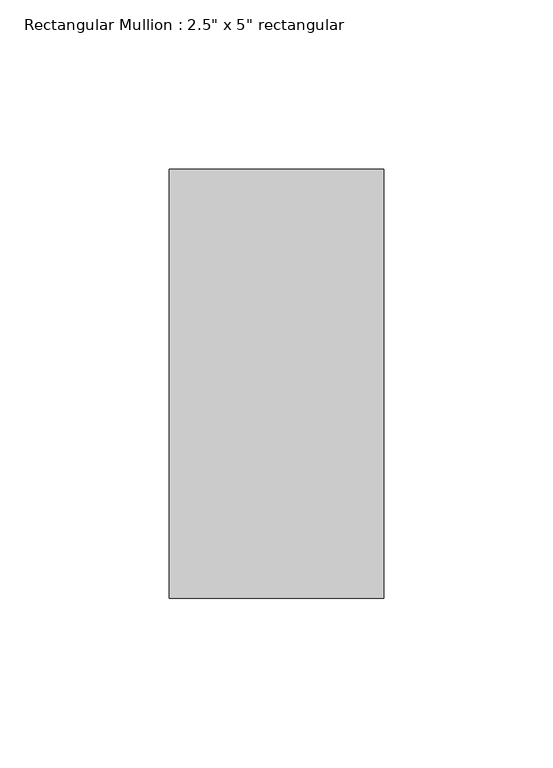
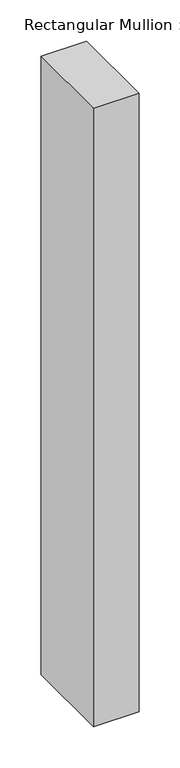
"""IFC4 building model written with IfcOpenShell, lengths in millimetres: member geometry."""

from ifc_helpers import new_model, si_unit, frame, origin, place, context, project, spatial, polyline, outline, extrude, source, transform, mapped, element, save


def member_73c23c35(model_context):
    return source(origin(), model_context, "Body", "SweptSolid", [
        extrude(outline(polyline([(0.0, 63.5), (0.0, -63.5), (-63.5, -63.5), (-63.5, 63.5), (0.0, 63.5)])), frame((0.0, 0.0, -914.4), z_axis=(0.0, 0.0, 1.0), x_axis=(1.0, 0.0, 0.0)), (0.0, 0.0, 1.0), 914.4),
    ])


if __name__ == "__main__":
    model = new_model("IFC4")
    model_context = context("Model", 3, world=origin())
    ifc_project = project(units=[si_unit("LENGTHUNIT", "METRE", prefix="MILLI")], contexts=[model_context])
    site = spatial("IfcSite", under=ifc_project)
    building = spatial("IfcBuilding", under=site)
    placement = place(None, origin())
    member_shape = member_73c23c35(model_context)
    element("IfcMember", 1, ObjectType="Rectangular Mullion : 2.5\" x 5\" rectangular", at=placement, inside=building, context=model_context, shape_type="MappedRepresentation", body=[
        mapped(member_shape, transform((0.0, 0.0, 0.0), x_axis=(1.0, 0.0, 0.0), y_axis=(0.0, 1.0, 0.0), z_axis=(0.0, 0.0, 1.0))),
    ])
    save(model, "model.ifc")

# Revit data of these elements
# Type "Rectangular Mullion : 2.5\" x 5\" rectangular"
#   built-in parameter 1007304 = 0.416667 (stored number, unit not read)
#   built-in parameter 1007301 = 0.104167 (stored number, unit not read)
#   built-in parameter 1007300 = 0.104167 (stored number, unit not read)
# Element 1 (IfcMember, "Rectangular Mullion : 2.5\" x 5\" rectangular")
#   Materials on its faces: "Aluminum"
# Materials
#   "Aluminum": class "Metal", colour RGB 247 247 247, transparency 0, Description = "Aluminum 6061", Cost = 0
